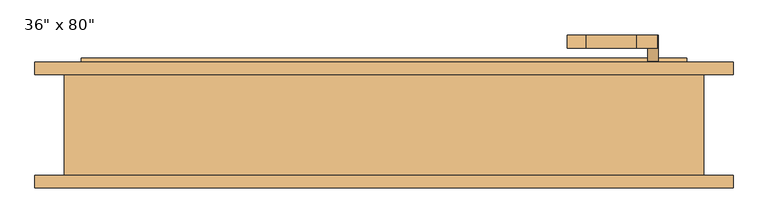
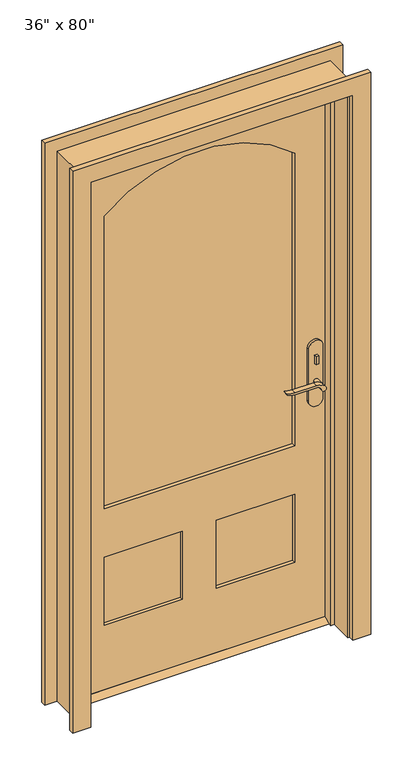
"""IFC4 building model written with IfcOpenShell, lengths in millimetres: door geometry."""

from ifc_helpers import new_model, si_unit, point, frame, frame_2d, origin, place, context, project, spatial, polyline, circle_curve, trimmed, segment, composite_curve, outline, extrude, faceted_brep, source, transform, mapped, element, save


def door_808aeb8e(model_context):
    return source(origin(), model_context, "Body", "SolidModel", [
        extrude(outline(polyline([(38.1, 12.7), (73.025, 12.7), (98.425, 0.0), (12.7, 0.0), (38.1, 12.7)])), frame((-457.2, 0.0, 0.0), z_axis=(1.0, 0.0, 0.0), x_axis=(0.0, 1.0, 0.0)), (0.0, 0.0, 1.0), 914.4),
        extrude(outline(polyline([(411.4, 18.1), (401.4, 18.1), (401.4, 28.1), (411.4, 28.1), (411.4, 18.1)])), frame((0.0, 0.0, 981.9), z_axis=(0.0, 0.0, 1.0), x_axis=(1.0, 0.0, 0.0)), (0.0, 0.0, 1.0), 30.0),
        extrude(outline(composite_curve([segment(trimmed(circle_curve(frame_2d((996.9, 406.4)), 8.0), [point((996.9, 398.4))], [point((996.9, 414.4))], False, "CARTESIAN"), True, "CONTINUOUS"), segment(trimmed(circle_curve(frame_2d((996.9, 406.4)), 8.0), [point((996.9, 414.4))], [point((996.9, 398.4))], False, "CARTESIAN"), True, "CONTINUOUS")], self_intersect=False)), frame((0.0, 83.025, 0.0), z_axis=(0.0, 1.0, 0.0), x_axis=(0.0, 0.0, 1.0)), (0.0, 0.0, 1.0), 10.0),
        extrude(outline(composite_curve([segment(trimmed(circle_curve(frame_2d((897.1555521, 382.7324871)), 37.2832219), [point((919.0523287, 412.9081363))], [point((934.4, 381.0325667))], False, "CARTESIAN"), True, "CONTINUOUS"), segment(polyline([(934.4, 381.0325667), (934.4, 304.7564091)]), True, "CONTINUOUS"), segment(trimmed(circle_curve(frame_2d((1017.6850638, 304.8227909)), 83.2850902), [point((934.4, 304.7564091))], [point((939.4, 276.4))], True, "CARTESIAN"), True, "CONTINUOUS"), segment(polyline([(939.4, 276.4), (936.6135558, 276.4)]), True, "CONTINUOUS"), segment(trimmed(circle_curve(frame_2d((986.6709207, 308.3396612)), 59.3791355), [point((936.6135558, 276.4))], [point((927.4, 304.7564091))], False, "CARTESIAN"), True, "CONTINUOUS"), segment(polyline([(927.4, 304.7564091), (927.4, 381.0138099)]), True, "CONTINUOUS"), segment(trimmed(circle_curve(frame_2d((909.2738613, 381.0138099)), 18.1261387), [point((927.4, 381.0138099))], [point((914.4, 398.4))], True, "CARTESIAN"), True, "CONTINUOUS"), segment(trimmed(circle_curve(frame_2d((914.4, 406.4)), 8.0), [point((914.4, 398.4))], [point((919.0523287, 412.9081363))], False, "CARTESIAN"), True, "CONTINUOUS")], self_intersect=False)), frame((0.0, -21.9, 0.0), z_axis=(0.0, 1.0, 0.0), x_axis=(0.0, 0.0, 1.0)), (0.0, 0.0, 1.0), 20.0),
        extrude(outline(composite_curve([segment(trimmed(circle_curve(frame_2d((914.4, 406.4)), 8.0), [point((914.3999903, 398.4))], [point((919.0523287, 412.9081363))], False, "CARTESIAN"), True, "CONTINUOUS"), segment(trimmed(circle_curve(frame_2d((897.1555521, 382.7324871)), 37.2832219), [point((919.0523287, 412.9081363))], [point((934.4, 381.0325667))], False, "CARTESIAN"), True, "CONTINUOUS"), segment(polyline([(934.4, 381.0325667), (934.4, 304.7564091)]), True, "CONTINUOUS"), segment(trimmed(circle_curve(frame_2d((1017.6850638, 304.8227909)), 83.2850902), [point((934.4, 304.7564091))], [point((939.4, 276.4))], True, "CARTESIAN"), True, "CONTINUOUS"), segment(polyline([(939.4, 276.4), (936.6135558, 276.4)]), True, "CONTINUOUS"), segment(trimmed(circle_curve(frame_2d((986.6709207, 308.3396612)), 59.3791355), [point((936.6135558, 276.4))], [point((927.4, 304.7564091))], False, "CARTESIAN"), True, "CONTINUOUS"), segment(polyline([(927.4, 304.7564091), (927.4, 381.0138122)]), True, "CONTINUOUS"), segment(trimmed(circle_curve(frame_2d((909.2738682, 381.0138122)), 18.1261318), [point((927.4, 381.0138122))], [point((914.3999903, 398.4))], True, "CARTESIAN"), True, "CONTINUOUS")], self_intersect=False)), frame((0.0, 113.025, 0.0), z_axis=(0.0, 1.0, 0.0), x_axis=(0.0, 0.0, 1.0)), (0.0, 0.0, 1.0), 20.0),
        extrude(outline(composite_curve([segment(trimmed(circle_curve(frame_2d((914.4, 406.4)), 8.0), [point((914.4, 398.4))], [point((914.4, 414.4))], False, "CARTESIAN"), True, "CONTINUOUS"), segment(trimmed(circle_curve(frame_2d((914.4, 406.4)), 8.0), [point((914.4, 414.4))], [point((914.4, 398.4))], False, "CARTESIAN"), True, "CONTINUOUS")], self_intersect=False)), frame((0.0, -1.9, 0.0), z_axis=(0.0, 1.0, 0.0), x_axis=(0.0, 0.0, 1.0)), (0.0, 0.0, 1.0), 30.0),
        extrude(outline(composite_curve([segment(trimmed(circle_curve(frame_2d((914.4, 406.4)), 8.0), [point((914.4, 398.4))], [point((914.4, 414.4))], False, "CARTESIAN"), True, "CONTINUOUS"), segment(trimmed(circle_curve(frame_2d((914.4, 406.4)), 8.0), [point((914.4, 414.4))], [point((914.4, 398.4))], False, "CARTESIAN"), True, "CONTINUOUS")], self_intersect=False)), frame((0.0, 83.025, 0.0), z_axis=(0.0, 1.0, 0.0), x_axis=(0.0, 0.0, 1.0)), (0.0, 0.0, 1.0), 30.0),
        extrude(outline(composite_curve([segment(polyline([(844.4, 431.4), (1039.4, 431.4)]), True, "CONTINUOUS"), segment(trimmed(circle_curve(frame_2d((1039.4, 406.4)), 25.0), [point((1039.4, 431.4))], [point((1039.4, 381.4))], False, "CARTESIAN"), True, "CONTINUOUS"), segment(polyline([(1039.4, 381.4), (844.4, 381.4)]), True, "CONTINUOUS"), segment(trimmed(circle_curve(frame_2d((844.4, 406.4)), 25.0), [point((844.4, 381.4))], [point((844.4, 431.4))], False, "CARTESIAN"), True, "CONTINUOUS")], self_intersect=False)), frame((0.0, 28.1, 0.0), z_axis=(0.0, 1.0, 0.0), x_axis=(0.0, 0.0, 1.0)), (0.0, 0.0, 1.0), 10.0),
        extrude(outline(composite_curve([segment(polyline([(844.4, 431.4), (1039.4, 431.4)]), True, "CONTINUOUS"), segment(trimmed(circle_curve(frame_2d((1039.4, 406.4)), 25.0), [point((1039.4, 431.4))], [point((1039.4, 381.4))], False, "CARTESIAN"), True, "CONTINUOUS"), segment(polyline([(1039.4, 381.4), (844.4, 381.4)]), True, "CONTINUOUS"), segment(trimmed(circle_curve(frame_2d((844.4, 406.4)), 25.0), [point((844.4, 381.4))], [point((844.4, 431.4))], False, "CARTESIAN"), True, "CONTINUOUS")], self_intersect=False)), frame((0.0, 73.025, 0.0), z_axis=(0.0, 1.0, 0.0), x_axis=(0.0, 0.0, 1.0)), (0.0, 0.0, 1.0), 10.0),
        extrude(outline(polyline([(2032.0, -457.2), (12.7, -457.2), (12.7, 457.2), (2032.0, 457.2), (2032.0, -457.2)]), holes=[composite_curve([segment(polyline([(688.975, -336.55), (1784.35, -336.55)]), True, "CONTINUOUS"), segment(trimmed(circle_curve(frame_2d((1401.92125, 0.0)), 509.42875), [point((1784.35, -336.55))], [point((1784.35, 336.55))], True, "CARTESIAN"), True, "CONTINUOUS"), segment(polyline([(1784.35, 336.55), (688.975, 336.55), (688.975, -336.55)]), True, "CONTINUOUS")], self_intersect=False), polyline([(508.0, -60.325), (254.0, -60.325), (254.0, -336.55), (508.0, -336.55), (508.0, -60.325)]), polyline([(508.0, 336.55), (254.0, 336.55), (254.0, 60.325), (508.0, 60.325), (508.0, 336.55)])]), frame((0.0, 38.1, 0.0), z_axis=(0.0, 1.0, 0.0), x_axis=(0.0, 0.0, 1.0)), (0.0, 0.0, 1.0), 34.925),
        faceted_brep([(482.6, 73.025, 0.0), (482.6, -79.375, 0.0), (457.2, -79.375, 0.0), (457.2, 3.175, 0.0), (444.5, 3.175, 0.0), (444.5, 38.1, 0.0), (457.2, 38.1, 0.0), (457.2, 73.025, 0.0), (482.6, 73.025, 2057.4), (482.6, -79.375, 2057.4), (-482.6, -79.375, 2057.4), (-482.6, -79.375, 0.0), (-457.2, -79.375, 0.0), (-457.2, -79.375, 2032.0), (457.2, -79.375, 2032.0), (457.2, 3.175, 2032.0), (-457.2, 3.175, 2032.0), (-457.2, 3.175, 0.0), (-444.5, 3.175, 0.0), (-444.5, 3.175, 2019.3), (444.5, 3.175, 2019.3), (444.5, 38.1, 2019.3), (-444.5, 38.1, 2019.3), (-444.5, 38.1, 0.0), (-457.2, 38.1, 0.0), (-457.2, 38.1, 2032.0), (457.2, 38.1, 2032.0), (457.2, 73.025, 2032.0), (-457.2, 73.025, 2032.0), (-457.2, 73.025, 0.0), (-482.6, 73.025, 0.0), (-482.6, 73.025, 2057.4)], [[[0, 1, 2, 3, 4, 5, 6, 7]], [[1, 0, 8, 9]], [[2, 1, 9, 10, 11, 12, 13, 14]], [[3, 2, 14, 15]], [[4, 3, 15, 16, 17, 18, 19, 20]], [[5, 4, 20, 21]], [[6, 5, 21, 22, 23, 24, 25, 26]], [[7, 6, 26, 27]], [[0, 7, 27, 28, 29, 30, 31, 8]], [[9, 8, 31, 10]], [[15, 14, 13, 16]], [[21, 20, 19, 22]], [[27, 26, 25, 28]], [[30, 29, 24, 23, 18, 17, 12, 11]], [[10, 31, 30, 11]], [[16, 13, 12, 17]], [[22, 19, 18, 23]], [[28, 25, 24, 29]]]),
        extrude(outline(polyline([(-60.325, 49.7416667), (-336.55, 49.7416667), (-336.55, 61.3833333), (-60.325, 61.3833333), (-60.325, 49.7416667)])), frame((0.0, 0.0, 254.0), z_axis=(0.0, 0.0, 1.0), x_axis=(1.0, 0.0, 0.0)), (0.0, 0.0, 1.0), 254.0),
        extrude(outline(polyline([(336.55, 49.7416667), (60.325, 49.7416667), (60.325, 61.3833333), (336.55, 61.3833333), (336.55, 49.7416667)])), frame((0.0, 0.0, 254.0), z_axis=(0.0, 0.0, 1.0), x_axis=(1.0, 0.0, 0.0)), (0.0, 0.0, 1.0), 254.0),
        extrude(outline(composite_curve([segment(polyline([(688.975, -336.55), (688.975, 336.55), (1784.35, 336.55)]), True, "CONTINUOUS"), segment(trimmed(circle_curve(frame_2d((1401.92125, 0.0)), 509.42875), [point((1784.35, 336.55))], [point((1784.35, -336.55))], False, "CARTESIAN"), True, "CONTINUOUS"), segment(polyline([(1784.35, -336.55), (688.975, -336.55)]), True, "CONTINUOUS")], self_intersect=False)), frame((0.0, 52.07, 0.0), z_axis=(0.0, 1.0, 0.0), x_axis=(0.0, 0.0, 1.0)), (0.0, 0.0, 1.0), 6.985),
        extrude(outline(polyline([(0.0, -527.05), (0.0, -463.55), (2038.35, -463.55), (2038.35, 463.55), (0.0, 463.55), (0.0, 527.05), (2101.85, 527.05), (2101.85, -527.05), (0.0, -527.05)])), frame((0.0, -98.425, 0.0), z_axis=(0.0, 1.0, 0.0), x_axis=(0.0, 0.0, 1.0)), (0.0, 0.0, 1.0), 19.05),
        extrude(outline(polyline([(0.0, -527.05), (0.0, -463.55), (2038.35, -463.55), (2038.35, 463.55), (0.0, 463.55), (0.0, 527.05), (2101.85, 527.05), (2101.85, -527.05), (0.0, -527.05)])), frame((0.0, 73.025, 0.0), z_axis=(0.0, 1.0, 0.0), x_axis=(0.0, 0.0, 1.0)), (0.0, 0.0, 1.0), 19.05),
    ])


if __name__ == "__main__":
    model = new_model("IFC4")
    model_context = context("Model", 3, world=origin())
    ifc_project = project(units=[si_unit("LENGTHUNIT", "METRE", prefix="MILLI")], contexts=[model_context])
    site = spatial("IfcSite", under=ifc_project)
    building = spatial("IfcBuilding", under=site)
    placement = place(None, origin())
    door_shape = door_808aeb8e(model_context)
    element("IfcDoor", 1, ObjectType="36\" x 80\"", at=placement, inside=building, context=model_context, shape_type="MappedRepresentation", body=[
        mapped(door_shape, transform((0.0, 0.0, 0.0), x_axis=(1.0, 0.0, 0.0), y_axis=(0.0, 1.0, 0.0), z_axis=(0.0, 0.0, 1.0))),
    ])
    save(model, "model.ifc")

# Revit data of these elements
# Type "36\" x 80\""
#   Type Mark = "8"
#   Assembly Code = "B2030100"
#   Analytic Construction = "French door, wood frame with single glass"
#   Threshold Offset [instance default] = 0' - 0 1/2"
#   Thickness = 0' - 1 3/8"
#   Thermal Resistance (R) = 1.0696 (h·ft²·°F)/BTU
#   Swing Angle [instance default] = 90.00°
#   Stiles = 0' - 4 3/4"
#   Rough Width = 3' - 2"
#   Rough Height = 6' - 9"
#   Radius = 1' - 8.05625"
#   Lock Rail = 0' - 7 1/8"
#   Height = 6' - 8"
#   Width = 3' - 0"
#   Heat Transfer Coefficient (U) = 0.9350 BTU/(h·ft²·°F)
#   Door Offset [instance default] = 0' - 0"
#   Bottom Rail = 0' - 9 1/2"
#   Threshold [instance default] = yes
#   Function = 1
#   Exterior Trim [instance default] = yes
#   Trim Material = Cherry
#   Threshold Material = Cherry
#   Panel Material = Cherry
#   Glazing = Glass
#   Frame Material = Cherry
#   Door Handle Material = Aluminum
#   Visual Light Transmittance = 0
#   Solar Heat Gain Coefficient = 0
#   Wall Closure = (empty or 0)
#   Construction Type = (empty or 0)
# Element 1 (IfcDoor, "36\" x 80\"")
#   Materials on its faces: "Cherry", "Aluminum", "Glass"
# Materials
#   "Cherry": class "Wood", colour RGB 226 177 128, transparency 0, Description = "Prunus Serotina", Cost = 0
#   "Glass": class "Glass", colour RGB 0 128 192, transparency 0.75, Description = "Soda Lime Glass", Cost = 0
#   "Aluminum": class "Metal", colour RGB 247 247 247, transparency 0, Description = "Aluminum 6061", Cost = 0
